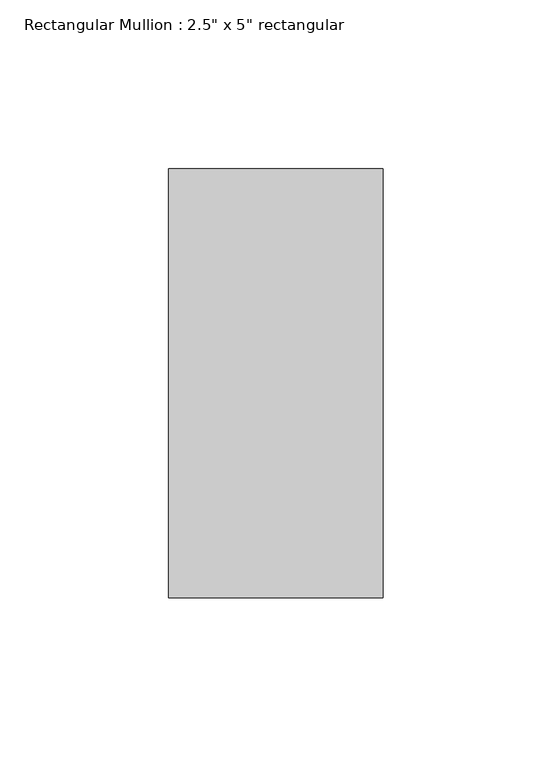
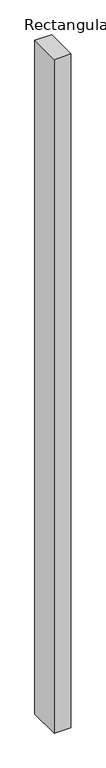
"""IFC4 building model written with IfcOpenShell, lengths in millimetres: member geometry."""

from ifc_helpers import new_model, si_unit, frame, origin, place, context, project, spatial, polyline, outline, extrude, source, transform, mapped, element, save


def member_e826b105(model_context):
    return source(origin(), model_context, "Body", "SweptSolid", [
        extrude(outline(polyline([(0.0, 63.5), (0.0, -63.5), (-63.5, -63.5), (-63.5, 63.5), (0.0, 63.5)])), frame((0.0, 0.0, -2717.8), z_axis=(0.0, 0.0, 1.0), x_axis=(1.0, 0.0, 0.0)), (0.0, 0.0, 1.0), 2717.8),
    ])


if __name__ == "__main__":
    model = new_model("IFC4")
    model_context = context("Model", 3, world=origin())
    ifc_project = project(units=[si_unit("LENGTHUNIT", "METRE", prefix="MILLI")], contexts=[model_context])
    site = spatial("IfcSite", under=ifc_project)
    building = spatial("IfcBuilding", under=site)
    placement = place(None, origin())
    member_shape = member_e826b105(model_context)
    element("IfcMember", 1, ObjectType="Rectangular Mullion : 2.5\" x 5\" rectangular", at=placement, inside=building, context=model_context, shape_type="MappedRepresentation", body=[
        mapped(member_shape, transform((0.0, 0.0, 0.0), x_axis=(1.0, 0.0, 0.0), y_axis=(0.0, 1.0, 0.0), z_axis=(0.0, 0.0, 1.0))),
    ])
    save(model, "model.ifc")

# Revit data of these elements
# Type "Rectangular Mullion : 2.5\" x 5\" rectangular"
#   built-in parameter 1007304 = 0.416667 (stored number, unit not read)
#   built-in parameter 1007301 = 0.104167 (stored number, unit not read)
#   built-in parameter 1007300 = 0.104167 (stored number, unit not read)
# Element 1 (IfcMember, "Rectangular Mullion : 2.5\" x 5\" rectangular")
#   Materials on its faces: "Iron, Ductile"
# Materials
#   "Iron, Ductile": class "Metal", colour RGB 0 0 0, transparency 0, Description = "Ductile cast iron", Cost = 0
